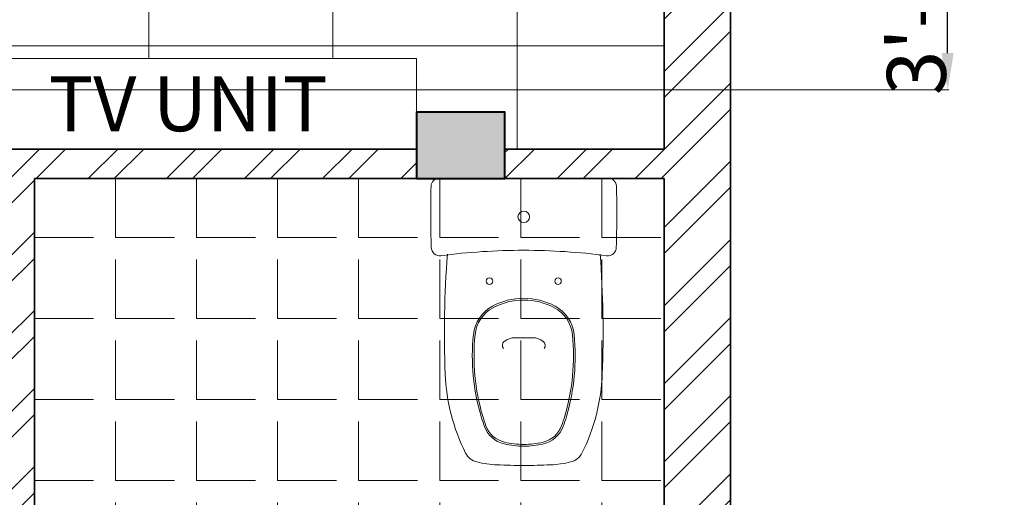
# Model space of a CAD drawing. Units: inches. Extents: x 351 to 1738, y -265 to 286.
# Tile 31 of 38: x 1470 to 1604, y -100 to -35. Entities that reach past the tile are written whole.
import ezdxf

# ---------------------------------------------------------------- set-up
doc = ezdxf.new("R2010")
doc.units = ezdxf.units.IN
doc.header["$MEASUREMENT"] = 0
for name, color, linetype, lineweight in [('A-ANNO-DIMS', 2, 'Continuous', 18), ('A-ANNO-TEXT', 7, 'Continuous', 18), ('A-COLS', 7, 'Continuous', 40), ('A-COLS-PATT', 6, 'Continuous', 13), ('A-FLOR-CASE', 9, 'Continuous', 18), ('A-FLOR-FIXT', 9, 'Continuous', 18), ('A-FLOR-PATT', 9, 'Continuous', 9), ('A-WALL', 7, 'Continuous', 35), ('A-WALL-PATT', 152, 'Continuous', 13)]:
    doc.layers.add(name, color=color, linetype=linetype, lineweight=lineweight)
doc.styles.add('Annotative', font='arial.ttf')
doc.styles.get("Standard").update_dxf_attribs({"font": 'arial.ttf'})
doc.dimstyles.get("Standard").update_dxf_attribs({"dimtxt": 8, "dimasz": 5, "dimexe": 0.18, "dimexo": 0.0625, "dimgap": 0.09, "dimtad": 1, "dimtoh": 1, "dimzin": 0, "dimdsep": 46, "dimlunit": 4, "dimtxsty": 'Standard', "dimcen": 0, "dimclre": 256, "dimadec": 0, "dimazin": 0, "dimtfac": 1, "dimtofl": 0, "dimtmove": 0, "dimatfit": 3, "dimfxl": 1, "dimtolj": 1, "dimtzin": 0, "dimlwe": -1, "dimarcsym": 0})

# ---------------------------------------------------------------- blocks, each defined once
blk = doc.blocks.new('A$C7E916B5A')
for p, q in [((0.019, 0.67), (0.2161, 0.67)), ((0.4133, 0.67), (0.2161, 0.67)), ((0.2161, 0.298), (0.1955, 0.298)), ((0.2161, 0.298), (0.2368, 0.298))]:
    blk.add_line(p, q)
for centre, radius in [((0.2161, 0.58), 0.0135), ((0.1361, 0.43), 0.0075), ((0.2961, 0.43), 0.0075)]:
    blk.add_circle(centre, radius)
for centre, radius, start, end in [((0.019, 0.651), 0.019, 90, 178.4999), ((0.4133, 0.651), 0.019, 1.5001, 90), ((2.5011, 0.586), 2.502, 178.4999, 181.7705), ((-2.0689, 0.586), 2.502, 358.2295, 1.5001), ((0.0203, 0.5093), 0.02, 181.7705, 277.4115), ((0.412, 0.5093), 0.02, 262.5885, 358.2295), ((0.2161, -0.996), 1.498, 90, 97.4115), ((2.5311, 0.3098), 2.5, 175.7895, 182.2108), ((0.2161, -0.996), 1.498, 82.5885, 90), ((-2.0989, 0.3098), 2.5, 357.7892, 4.2105), ((0.1832, 0.2967), 0.085, 118.1012, 174.3336), ((0.1832, 0.2967), 0.081, 118.1012, 174.3336), ((0.2161, 0.235), 0.155, 90, 118.1012), ((0.2161, 0.235), 0.151, 90, 118.1012), ((0.2161, 0.235), 0.155, 61.8988, 90), ((0.2161, 0.235), 0.151, 61.8988, 90), ((0.2491, 0.2967), 0.081, 5.6664, 61.8988), ((0.2491, 0.2967), 0.085, 5.6664, 61.8988), ((0.5961, 0.2558), 0.5, 174.3336, 196.4495), ((0.5961, 0.2558), 0.496, 174.3336, 196.4495), ((-0.1639, 0.2558), 0.496, 343.5505, 5.6664), ((-0.1639, 0.2558), 0.5, 343.5505, 5.6664), ((0.1781, 0.28), 0.012, 128.2132, 217.5723), ((0.1955, 0.258), 0.04, 90, 128.2132), ((0.2368, 0.258), 0.04, 51.7868, 90), ((0.2541, 0.28), 0.012, 322.4277, 51.7868), ((0.4827, 0.2307), 0.45, 182.2108, 206.6241), ((-0.0504, 0.2307), 0.45, 333.3759, 357.7892), ((0.4811, 0.2218), 0.376, 196.4495, 200.1007), ((-0.0488, 0.2218), 0.376, 339.8993, 343.5505), ((0.4811, 0.2218), 0.38, 196.4495, 200.1007), ((0.1851, 0.1135), 0.0609, 200.1007, 256.7352), ((0.2471, 0.1135), 0.0609, 283.2648, 339.8993), ((-0.0488, 0.2218), 0.38, 339.8993, 343.5505), ((0.1851, 0.1135), 0.0649, 200.1007, 256.7352), ((0.2471, 0.1135), 0.0649, 283.2648, 339.8993), ((0.2161, 0.245), 0.2, 256.7352, 270), ((0.2161, 0.245), 0.196, 256.7352, 270), ((0.2161, 0.245), 0.196, 270, 283.2648), ((0.2161, 0.245), 0.2, 270, 283.2648), ((0.1161, 0.047), 0.04, 206.6241, 256.4771), ((0.3161, 0.047), 0.04, 283.5229, 333.3759), ((0.1652, 0.2512), 0.25, 256.477, 267.3481), ((0.2161, 1.35), 1.35, 267.3481, 270), ((0.2161, 1.35), 1.35, 270, 272.6519), ((0.267, 0.2512), 0.25, 272.6519, 283.523)]:
    blk.add_arc(centre, radius, start, end)
blk = doc.blocks.new('CONSOLE-TV')
blk.add_lwpolyline([(0, 0), (61, 0), (61, 12.29), (0, 12.29)], close=True)
blk = doc.blocks.new('COL-9x12')
blk.add_lwpolyline([(0, 12), (0, 0), (9, 0), (9, 12)], close=True)
blk = doc.blocks.new('*D66')
at = {"layer": 'A-ANNO-DIMS', "transparency": 16777216}
for p, q in [((1384.27, -3.5), (1596.33, -3.5)), ((1384.27, -45), (1596.33, -45))]:
    blk.add_line(p, q, dxfattribs=at)
at = {"layer": 'A-ANNO-DIMS', "color": 0, "lineweight": -2, "transparency": 16777216}
blk.add_line((1596.15, -40), (1596.15, -8.5), dxfattribs=at)
at = {"layer": 'A-ANNO-DIMS', "color": 0, "transparency": 16777216}
for points in [[(1595.32, -8.5), (1596.99, -8.5), (1596.15, -3.5)], [(1595.32, -40), (1596.99, -40), (1596.15, -45)]]:
    blk.add_solid(points, dxfattribs=at)
at = {"layer": 'Defpoints', "color": 0, "transparency": 16777216}
for p in [(1384.2, -3.5), (1596.15, -3.5), (1384.2, -45)]:
    blk.add_point(p, dxfattribs=at)
at = {"layer": 'A-ANNO-DIMS', "color": 0, "transparency": 16777216, "insert": (1591.92, -24.25), "char_height": 8, "attachment_point": 5, "rotation": 90}
blk.add_mtext('\\A1;3\'-5 1/2"', dxfattribs=at)

msp = doc.modelspace()

# ---------------------------------------------------------------- hatches: boundary and pattern name
at = {"layer": 'A-COLS-PATT'}
h = msp.add_hatch(color=256, dxfattribs=at)
h.dxf.hatch_style = 1
h.paths.add_polyline_path([(1112.704, 237.963), (1103.704, 237.963), (1103.704, 228.963), (1112.704, 228.963)])
h.paths.add_polyline_path([(1115.704, 237.963), (1112.704, 237.963), (1112.704, 228.963), (1115.704, 228.963)])
h.paths.add_polyline_path([(1043.704, 255.963), (1034.704, 255.963), (1034.704, 243.963), (1043.704, 243.963)])
h.paths.add_polyline_path([(1043.704, 210.963), (1034.704, 210.963), (1034.704, 198.963), (1043.704, 198.963)])
h.paths.add_polyline_path([(1043.704, -45.037), (1034.704, -45.037), (1034.704, -57.037), (1043.704, -57.037)])
h.paths.add_polyline_path([(1112.704, -45.037), (1103.704, -45.037), (1103.704, -57.037), (1112.704, -57.037)])
h.paths.add_polyline_path([(1112.704, -161.037), (1103.704, -161.037), (1103.704, -164.037), (1103.704, -173.037), (1112.704, -173.037)])
h.paths.add_polyline_path([(1043.704, -161.037), (1034.704, -161.037), (1034.704, -173.037), (1043.704, -173.037)])
h.paths.add_polyline_path([(1248.549, -164.037), (1236.549, -164.037), (1236.549, -173.037), (1248.549, -173.037)])
h.paths.add_polyline_path([(1248.549, -50), (1236.549, -50), (1236.549, -59), (1248.549, -59)])
h.paths.add_polyline_path([(1248.704, 73.463), (1244.704, 73.463), (1244.704, 64.463), (1248.704, 64.463)])
h.paths.add_polyline_path([(1244.704, 73.463), (1236.704, 73.463), (1236.704, 64.463), (1244.704, 64.463)])
h.paths.add_polyline_path([(1248.704, 237.963), (1236.704, 237.963), (1236.704, 228.963), (1248.704, 228.963)])
h.paths.add_polyline_path([(1392.204, 237.963), (1380.204, 237.963), (1380.204, 228.963), (1392.204, 228.963)])
h.paths.add_polyline_path([(1536.064, 237.963), (1524.064, 237.963), (1524.064, 228.963), (1536.064, 228.963)])
h.paths.add_polyline_path([(1536.064, 73.463), (1524.064, 73.463), (1524.064, 64.463), (1536.064, 64.463)])
h.paths.add_polyline_path([(1384.204, 73.463), (1380.204, 73.463), (1380.204, 64.463), (1384.204, 64.463)])
h.paths.add_polyline_path([(1392.064, 73.463), (1384.204, 73.463), (1384.204, 64.463), (1392.064, 64.463)])
h.paths.add_polyline_path([(1536.064, -53.037), (1524.064, -53.037), (1524.064, -57.037), (1536.064, -57.037)])
h.paths.add_polyline_path([(1536.064, -48.037), (1524.064, -48.037), (1524.064, -53.037), (1536.064, -53.037)])
h.paths.add_polyline_path([(1392.064, -48.037), (1380.064, -48.037), (1380.064, -56.5), (1380.065, -57.037), (1392.064, -57.037)])
h.paths.add_polyline_path([(1536.064, -164.037), (1524.064, -164.037), (1524.064, -173.037), (1536.064, -173.037)])
at = {"layer": 'A-FLOR-PATT', "transparency": 33554559}
h = msp.add_hatch(dxfattribs=at)
h.set_pattern_fill('ANSI37', color=256, scale=200, angle=135)
h.set_pattern_definition([(180, (1112.704, -164.037), (-2e-15, -25), []), (270, (1112.704, -164.037), (25, -5e-15), [])])
h.paths.add_polyline_path([(1380.064, 73.463), (1380.132, 148.463), (1338.064, 148.463), (1290.704, 148.463), (1290.704, 88.463), (1248.704, 88.463), (1248.704, -2.009), (1244.704, -2.009), (1244.704, 142.457), (1160.704, 142.457), (1160.704, 158.963), (1160.704, 170.137), (1160.704, 206.137), (1160.704, 228.963), (1112.704, 228.963), (1112.704, 209.963), (1112.704, 168.963), (1124.704, 168.963), (1124.704, 162.963), (1112.704, 162.963), (1112.704, 64.463), (1112.704, 60.463), (1112.704, 0.463), (1112.704, -48.026), (1146.804, -47.981), (1146.804, -35.691), (1207.804, -35.691), (1207.804, -47.902), (1236.542, -47.864), (1236.544, -50.009), (1248.5, -50.009), (1248.506, -102.915), (1248.512, -150.915), (1248.514, -164.037), (1248.549, -164.037), (1273.017, -164.037), (1273.017, -128.799), (1355.24, -128.799), (1355.24, -164.037), (1384.204, -164.037), (1384.204, -57.037), (1380.064, -57.037), (1380.064, -48.037), (1392.064, -48.037), (1392.064, -53.037), (1406.549, -53.037), (1406.549, -57.037), (1401.204, -57.037), (1401.204, -147.037), (1468.204, -147.037), (1468.204, -138.5), (1472.204, -138.5), (1472.204, -102.5), (1468.204, -102.5), (1468.204, -57.037), (1442.549, -57.037), (1442.549, -53.037), (1463.049, -53.037), (1463.049, -40.747), (1524.049, -40.747), (1524.049, -48.037), (1536.064, -48.037), (1536.064, -53.037), (1557.704, -53.037), (1557.704, 204.963), (1384.204, 204.963), (1384.204, 73.463), (1392.064, 73.463), (1392.064, 64.463), (1384.204, 64.463), (1384.204, -3.5), (1380.204, -3.537), (1380.204, 64.463), (1380.064, 64.463)])
h.paths.add_polyline_path([(1510.714, 86.458, -0.1039845), (1511.661, 85.595, 0.4704384), (1510.158, 87.614, 0.0961001)], flags=16)
h.paths.add_polyline_path([(1510.443, 100.266, 0.009798), (1504.693, 100.48, 0.0287898), (1504.6, 99.767, -0.1653311), (1505.519, 96.135, -0.1436014)], flags=16)
h.paths.add_polyline_path([(1487.201, 85.595, -0.1039845), (1488.148, 86.458, 0.0961001), (1488.704, 87.614, 0.4704384)], flags=0)
h.paths.add_polyline_path([(1495.052, 100.43), (1494.178, 100.43, -0.0264629), (1494.262, 99.774, -0.1442193)], flags=16)
h.paths.add_polyline_path([(1444.485, 86.458, -0.1039845), (1445.433, 85.595, 0.4704384), (1443.93, 87.614, 0.0961001)], flags=16)
h.paths.add_polyline_path([(1420.972, 85.595, -0.1039845), (1421.92, 86.458, 0.0961001), (1422.475, 87.614, 0.4704384)], flags=16)
h.paths.add_polyline_path([(1428.632, 100.335, 0.0010541), (1427.971, 100.309, -0.0215241), (1428.033, 99.774, -0.1143008)], flags=16)
h.paths.add_polyline_path([(1419.906, 143.708, 0.0249793), (1420.222, 157.526), (1421.573, 159.101), (1421.573, 175.369), (1391.393, 175.369), (1391.393, 200.519), (1542.294, 200.519), (1542.294, 175.369), (1512.028, 175.369, 0.0198653), (1511.521, 153.838, 0.0251335), (1512.758, 118.323, 0.0205529), (1512.942, 115.253), (1419.834, 115.253, -0.0004142), (1419.843, 124.798), (1413.059, 124.798), (1413.059, 84.437, -0.0618528), (1415.831, 80.45, -0.0930773), (1420.972, 85.595, -0.2675367), (1422.371, 84.732, 0.0851103), (1424.052, 84.616, -0.8853927), (1424.033, 84.851, -1.1258145), (1424.073, 84.366, -0.0879871), (1422.371, 84.732, -0.2675367), (1422.326, 83.089, -0.3705421), (1420.972, 85.595, 0.0930773), (1415.831, 80.45, -0.0874142), (1417.914, 73.937), (1418.941, 73.937, 0.0272504), (1418.913, 76.906, -0.1157032), (1421.051, 73.937), (1445.354, 73.937, -0.1157032), (1447.492, 76.906, 0.0272504), (1447.464, 73.937), (1448.491, 73.937, -0.0874142), (1450.574, 80.45, 0.0930773), (1445.433, 85.595, -0.3705421), (1444.079, 83.089, -0.2675367), (1444.034, 84.732, -0.0879871), (1442.332, 84.366, -1.1258145), (1442.372, 84.851, -2.0327363), (1442.364, 84.368, 0.0863779), (1444.034, 84.732, -0.2675367), (1445.433, 85.595, -0.0930773), (1450.574, 80.45, -0.2577317), (1466.483, 90.927, -0.4786702), (1468.832, 91.907, -0.4786702), (1471.18, 90.927, -0.26264), (1483.053, 81.78, -0.0718662), (1487.201, 85.595, -0.2675367), (1488.6, 84.732, 0.0851103), (1490.28, 84.616, -0.8853927), (1490.262, 84.851, -1.1258145), (1490.301, 84.366, -0.0879871), (1488.6, 84.732, -0.2675367), (1488.554, 83.089, -0.3705421), (1487.201, 85.595, 0.0718662), (1483.053, 81.78, -0.1320648), (1484.143, 73.937), (1485.169, 73.937, 0.0272504), (1485.142, 76.906, -0.1157032), (1487.28, 73.937), (1511.582, 73.937, -0.1157032), (1513.72, 76.906, 0.0272504), (1513.693, 73.937), (1514.719, 73.937, -0.0874142), (1516.802, 80.45, 0.0930773), (1511.661, 85.595, -0.3705421), (1510.308, 83.089, -0.2675367), (1510.262, 84.732, -0.0879871), (1508.561, 84.366, -1.1258145), (1508.601, 84.851, -2.0327363), (1508.592, 84.368, 0.0863779), (1510.262, 84.732, -0.2675367), (1511.661, 85.595, -0.0930773), (1516.802, 80.45, -0.0618528), (1519.575, 84.437), (1519.575, 73.937), (1413.059, 73.937), (1413.059, 124.798), (1419.843, 124.798, -0.0008205)], flags=16)
h.paths.add_polyline_path([(1220.149, 54.133, -0.1039845), (1220.869, 53.476, 0.4704384), (1219.727, 55.011, 0.0961001)], flags=16)
h.paths.add_polyline_path([(1219.944, 64.626, 0.009798), (1215.574, 64.789, 0.0287898), (1215.503, 64.247, -0.1653311), (1216.201, 61.487, -0.1436014)], flags=16)
h.paths.add_polyline_path([(1209.779, 64.449, 0.0974459), (1209.339, 64.751), (1208.247, 64.751, 0.1273905), (1207.7, 64.326, 0.1715858), (1206.95, 61.475, -0.1588542), (1207.636, 59.45, 0.0158984), (1207.795, 59.218, 0.0615457), (1208.598, 59.616, 0.1754158), (1208.638, 60.099, -0.2847793), (1209.348, 62.472, 0.3262165)], flags=16)
h.paths.add_polyline_path([(1169.818, 54.133, -0.1039845), (1170.538, 53.476, 0.4704384), (1169.396, 55.011, 0.0961001)], flags=16)
h.paths.add_polyline_path([(1159.017, 62.472, 0.2847642), (1158.307, 60.099, -0.1754332), (1158.267, 59.616, 0.3929302), (1159.448, 64.449, -0.3262298)], flags=16)
h.paths.add_polyline_path([(1156.342, 58.239, -0.1783213), (1154.011, 55.31, -0.1747359), (1154.722, 55.233, -0.2008015), (1156.27, 56.086, 0.1269899), (1157.283, 58.991, -0.0912053)], flags=16)
h.paths.add_polyline_path([(1156.624, 61.413, 0.1572752), (1157.316, 64.247, 0.1696217)], flags=16)
h.paths.add_polyline_path([(1152.67, 54.133, -0.0961001), (1151.95, 53.476, 0.0640762), (1154.465, 54.384, 0.1990158)], flags=16)
h.paths.add_polyline_path([(1202.281, 53.476, -0.1039845), (1203, 54.133, 0.0961001), (1203.423, 55.011, 0.4704384)], flags=0)
h.paths.add_polyline_path([(1151.139, 97.64, 0.0249793), (1151.379, 108.141), (1152.406, 109.338), (1152.406, 121.701), (1129.47, 121.701), (1129.47, 140.814), (1244.149, 140.814), (1244.149, 121.701), (1221.148, 121.701, 0.0198653), (1220.763, 105.338, 0.0251335), (1221.703, 78.349, 0.0205529), (1221.843, 76.016), (1151.078, 76.016, -0.1287433), (1148.786, 65.037, 0.5393525), (1150.327, 64.171, -0.027594), (1163.481, 64.751, 0.0976954), (1163.04, 64.449, 0.3262165), (1163.471, 62.472, -0.2847765), (1164.181, 60.099, -0.1947567), (1165.846, 61.443, -0.1554021), (1165.172, 64.247, -0.1660224), (1165.869, 61.475, -0.1770142), (1167.852, 62.77, -0.4482027), (1169.974, 60.807, -0.3934987), (1167.679, 57.86, -0.8955483), (1168.438, 54.524, -0.3557668), (1166.218, 56.086, -0.066024), (1165.505, 57.539), (1165.251, 56.243, -0.3717324), (1164.02, 59.758, -0.3736141), (1163.04, 64.449, -0.0976954), (1163.481, 64.751, 0.0213538), (1153.294, 64.429, -0.1341826), (1156.695, 61.368, 0.1868727), (1154.636, 62.77, 0.4482027), (1152.514, 60.807, 0.4037263), (1154.905, 57.846, 0.7112192), (1153.334, 55, 0.5315397), (1151.95, 53.476, -0.2675367), (1153.013, 52.821, 0.0851103), (1154.29, 52.732, -0.8853927), (1154.276, 52.911, -1.1258145), (1154.306, 52.543, -0.0879871), (1153.013, 52.821, -0.2675367), (1152.978, 51.572, -0.3705421), (1151.95, 53.476, 0.0930773), (1148.043, 49.566, -0.0874142), (1149.626, 44.617), (1150.406, 44.617, 0.0272504), (1150.385, 46.873, -0.1157032), (1152.01, 44.617), (1170.478, 44.617, -0.1157032), (1172.103, 46.873, 0.0272504), (1172.082, 44.617), (1172.862, 44.617, -0.0874142), (1174.445, 49.566, 0.0930773), (1170.538, 53.476, -0.3705421), (1169.51, 51.572, -0.2675367), (1169.475, 52.821, -0.0879871), (1168.182, 52.543, -1.1258145), (1168.212, 52.911, -2.0327363), (1168.206, 52.544, 0.0863779), (1169.475, 52.821, -0.2675367), (1170.538, 53.476, -0.0930773), (1174.445, 49.566, -0.2577317), (1186.536, 57.528, -0.4786702), (1188.321, 58.273, -0.4786702), (1190.106, 57.528, -0.26264), (1199.128, 50.577, -0.0718662), (1202.281, 53.476, -0.2675367), (1203.344, 52.821, 0.0851103), (1204.621, 52.732, -0.8853927), (1204.607, 52.911, -1.1258145), (1204.637, 52.543, -0.0879871), (1203.344, 52.821, -0.2675367), (1203.309, 51.572, -0.3705421), (1202.281, 53.476, 0.0718662), (1199.128, 50.577, -0.1320648), (1199.957, 44.617), (1200.737, 44.617, 0.0272504), (1200.716, 46.873, -0.1157032), (1202.341, 44.617), (1220.809, 44.617, -0.1157032), (1222.434, 46.873, 0.0272504), (1222.413, 44.617), (1223.193, 44.617, -0.0874142), (1224.776, 49.566, 0.0930773), (1220.869, 53.476, -0.3705421), (1219.841, 51.572, -0.2675367), (1219.806, 52.821, -0.0879871), (1218.513, 52.543, -1.1258145), (1218.543, 52.911, -2.0327363), (1218.537, 52.544, 0.0863779), (1219.806, 52.821, -0.2675367), (1220.869, 53.476, -0.0930773), (1224.776, 49.566, -0.0618528), (1226.883, 52.597), (1226.883, 44.617), (1145.936, 44.617), (1145.936, 83.269), (1151.091, 83.269, -0.0008205)], flags=16)
h.paths.add_polyline_path([(1218.01, 57.86, -0.8955483), (1218.769, 54.524, -0.3557668), (1216.549, 56.086, -0.066024), (1215.836, 57.539), (1215.582, 56.243, -0.3717324), (1214.351, 59.758, -0.3736141), (1213.371, 64.449, 0.3262165), (1213.802, 62.472, -0.2847765), (1214.512, 60.099, -0.1947567), (1216.177, 61.443, -0.1799907), (1218.183, 62.77, -0.4482027), (1220.305, 60.807, -0.3934987)], flags=16)
h.paths.add_polyline_path([(1424.735, 91.363, -0.3934987), (1421.715, 95.241, -0.4482027), (1424.507, 97.824, -0.1799907), (1427.147, 96.077, -0.1947567), (1429.338, 94.309, -0.2847765), (1430.272, 97.432, 0.3262165), (1430.839, 100.034, -0.3736141), (1429.55, 93.861, -0.3717324), (1427.929, 89.235), (1427.596, 90.941, -0.066024), (1426.657, 89.029, -0.3557668), (1423.736, 86.973, -0.8955483)], flags=16)
h.paths.add_polyline_path([(1238.033, 131.257, -1), (1227.329, 131.257, -1)], flags=0)
h.paths.add_polyline_path([(1235.357, 131.257, -1), (1230.005, 131.257, -1)], flags=0)
h.paths.add_polyline_path([(1214.039, 54.243, 0.1543819), (1214.38, 53.992, 0.3589549), (1213.613, 54.016, 0.6039484), (1214.379, 53.657, 0.3713191), (1213.968, 52.872, 0.1879935), (1214.312, 52.809, -0.592455), (1213.953, 52.967, -0.2942791), (1214.083, 53.691, -1.3001871), (1213.881, 54.134, -0.2837621), (1214.469, 53.896, 1.1509396)], flags=16)
h.paths.add_polyline_path([(1212.091, 56.286, -0.4084338), (1211.337, 56.445, -0.0362594), (1211.098, 56.848, -0.2360976), (1211.59, 56.63, 0.0353445), (1211.835, 56.543, -0.4752408), (1212.091, 56.286, -0.4752408), (1212.438, 56.182, 0.0353445), (1212.631, 56.007, -0.2360976), (1213.056, 55.676, -0.0362594), (1212.588, 55.697, -0.4084338)], flags=16)
h.paths.add_polyline_path([(1211.469, 50.297, 0.296043), (1210.47, 50.527, 0.310883), (1211.931, 50.148, 0.0212546)], flags=16)
h.paths.add_polyline_path([(1213.739, 51.818, -0.0362594), (1213.271, 51.838, -0.4084337), (1212.774, 52.427, -0.0947856), (1212.293, 50.703, 1.1504738), (1212.911, 50.232, 0.1662877), (1213.265, 50.68, -0.0252543), (1212.603, 50.13, 1.0879317), (1212.471, 49.407, 0.1662877), (1213.02, 49.251, -0.016128), (1212.567, 49.563, -0.286859), (1212.217, 49.638, 0.0221563), (1212.046, 50.055, -0.6461302), (1212.185, 50.498, 0.0884116), (1212.732, 52.077, -1.1860374), (1213.121, 52.323, 0.0353445), (1213.314, 52.148, -0.2360976)], flags=16)
h.paths.add_polyline_path([(1212.094, 50.342, -0.0485241), (1211.54, 49.605, -1.1038339), (1211.397, 48.738, -0.7855147), (1211.683, 48.254, -0.3920429), (1210.948, 48.525, -0.3928194), (1210.561, 47.995, -0.592455), (1210.201, 48.153, -0.2942791), (1210.331, 48.877, -0.7041716), (1210.316, 49.592, -0.6793441), (1210.729, 50.112, 0.5636764)], flags=16)
h.paths.add_polyline_path([(1211.274, 49.829, -0.1398258), (1210.745, 49.859, -0.2178785), (1210.948, 49.509, -0.4985724)], flags=0)
h.paths.add_polyline_path([(1433.426, 81.49, -0.181571), (1434.245, 81.788, -0.0080665), (1433.726, 82.205, 0.0455784), (1432.755, 81.242, 0.1790113)], flags=16)
h.paths.add_polyline_path([(1434.146, 81.009, -0.1324418), (1433.645, 80.771, 0.2590893), (1433.234, 80.471, -0.1802109), (1433.392, 80.805, -0.1699398), (1432.758, 81.109, 0.0326525), (1433.273, 80.474, -0.4933627), (1434.046, 80.146, -0.3904966)], flags=16)
h.paths.add_polyline_path([(1434.83, 80.047, -0.9475376), (1435.294, 79.576, -0.2991282), (1434.625, 79.404, -0.2704392), (1435.01, 78.591, -0.592455), (1434.537, 78.382, -0.3928194), (1434.027, 79.08, -0.3920429), (1433.06, 78.723, -0.3520423), (1433.003, 79.197, -0.1972159), (1433.75, 79.734, -0.7136405), (1434.447, 79.939, -0.2147903), (1434.819, 80.475, 0.4088333), (1435.075, 80.803, -0.2261519)], flags=16)
h.paths.add_polyline_path([(1432.67, 81.217, -0.4542182), (1431.897, 79.923, -0.4144105), (1431.301, 80.035, 0.0161291), (1431.897, 80.445, 0.2795702), (1432.073, 80.871, -0.2895037), (1431.103, 81.321, -0.4144105), (1430.978, 81.915, 0.0161296), (1431.586, 81.521, 0.341293), (1432.125, 81.583, -0.8131856)], flags=16)
h.paths.add_polyline_path([(1429.893, 86.381, -0.9475376), (1430.358, 85.91, -0.1731062), (1429.984, 85.712, -0.0388172), (1431.625, 84.214, -0.0879005), (1432.097, 88.549, -0.0497684), (1431.254, 88.49, -0.2360976), (1431.814, 88.925, 0.0353445), (1432.067, 89.155, -0.4752408), (1432.524, 89.291, -0.4752408), (1432.86, 89.63, 0.0353445), (1433.182, 89.744, -0.2360976), (1433.83, 90.032, -0.0362594), (1433.516, 89.502, -0.4084338), (1432.524, 89.291, -0.3124239), (1432.106, 88.58, 0.0885594), (1431.625, 84.214, -0.4084337), (1430.971, 83.439, -0.0362594), (1430.355, 83.412, -0.2360976), (1430.914, 83.847, 0.0353445), (1431.168, 84.078, -0.4752408), (1431.625, 84.214, 0.0388172), (1429.984, 85.712, -0.3217316), (1429.333, 86.048, -0.32743), (1429.883, 86.809, 0.4088333), (1430.138, 87.138, -0.2261519)], flags=16)
h.paths.add_polyline_path([(1211.206, 58.616, -0.9997836), (1211.336, 59.323, -0.6149935)], flags=16)
h.paths.add_polyline_path([(1210.288, 49.429, 0.1543819), (1210.629, 49.178, 0.3589549), (1209.861, 49.202, 0.6039484), (1210.627, 48.843, -0.5348247), (1210.806, 49.295, 0.7483464)], flags=16)
h.paths.add_polyline_path([(1209.589, 51.828, -0.0087906), (1209.775, 51.753, 0.1122315), (1209.466, 52.019, 1.4188509), (1209.014, 51.708, -0.4587257), (1208.651, 51.073, -0.592455), (1208.291, 51.232, -0.2942791), (1208.421, 51.955, -1.3001871), (1208.219, 52.398, -0.2260052), (1208.719, 52.257, -0.4755189), (1209.158, 52.369, -1.4554994), (1209.603, 52.664, 0.4213049), (1209.191, 52.262, -0.5912116), (1208.979, 51.796, 0.4973986), (1209.773, 51.333, 0.6493116)], flags=16)
h.paths.add_polyline_path([(1208.029, 52.041, 0.5446671), (1208.832, 52.045, 0.220132)], flags=0)
h.paths.add_polyline_path([(1210.438, 51.425, -0.2041997), (1210.277, 52.018, 0.2708262), (1209.915, 52.897, 0.3241145)], flags=0)
h.paths.add_polyline_path([(1209.668, 52.407, -0.60139), (1208.99, 52.221, -0.3949159), (1208.248, 52.83, -0.8367916), (1208.651, 53.017, -0.3384876), (1209.039, 52.571, 0.1941379), (1209.191, 52.262, 0.4139945), (1209.712, 52.475, 0.5177103), (1210.503, 51.416, 0.401922), (1209.493, 50.93, 0.2063956), (1209.516, 50.165, -0.3194629), (1210.417, 51.418, -0.466635)], flags=16)
h.paths.add_polyline_path([(1206.601, 56.086, -0.3557668), (1204.381, 54.524, -0.9211983), (1205.236, 57.846, 0.2065693), (1207.614, 58.991, -0.1269899)], flags=16)
h.paths.add_polyline_path([(1435.487, 82.816, 0.5277653), (1436.615, 83.361, 0.5085402), (1437.05, 82.433, 0.592455), (1437.524, 82.641, 0.3312448), (1436.963, 83.548, 0.3878632), (1437.808, 83.626, 0.5929544), (1437.618, 84.176, 0.2260158), (1436.961, 83.99, 0.3182053), (1437.588, 84.854, 0.6893744), (1437.05, 84.991, 0.3357648), (1436.539, 84.41, -0.1569934), (1436.404, 84.065, -0.4346112), (1436.961, 83.99, -0.2147903), (1437.333, 84.526, 0.4088333), (1437.588, 84.854, -0.2261519), (1437.343, 84.097, -0.9475376), (1437.808, 83.626, -0.2991282), (1437.139, 83.455, -0.2704392), (1437.524, 82.641, -0.592455), (1437.05, 82.433, -0.3928194), (1436.541, 83.13, -0.4396601), (1435.475, 82.794, -0.174614), (1435.942, 82.244, -0.2063956), (1435.912, 81.237, -0.2708262), (1435.125, 82.208, 0.2079765), (1434.686, 82.904, -0.1964955)], flags=16)
h.paths.add_polyline_path([(1435.386, 84.832, 0.270811), (1434.91, 83.676, -0.2042174), (1434.699, 82.895, 0.3241145)], flags=0)
h.paths.add_polyline_path([(1435.68, 84.18, -0.2176564), (1435.554, 83.304, -0.1767045), (1436.236, 83.778, -0.3730364)], flags=0)
h.paths.add_polyline_path([(1435.566, 100.034, 0.3262165), (1436.133, 97.432, -0.2847765), (1437.067, 94.309, -0.1947567), (1439.258, 96.077, -0.1554021), (1438.371, 99.767, -0.1660224), (1439.289, 96.12, -0.1770142), (1441.897, 97.824, -0.4482027), (1444.69, 95.241, -0.3934987), (1441.67, 91.363, -0.8955483), (1442.669, 86.973, -0.3557668), (1439.748, 89.029, -0.066024), (1438.809, 90.941), (1438.476, 89.235, -0.3717324), (1436.855, 93.861, -0.3736141)], flags=16)
h.paths.add_polyline_path([(1191.252, 49.507, -0.2740221), (1190.658, 48.409, 0.2675367), (1191.311, 47.344, 0.3705421)], flags=0)
h.paths.add_polyline_path([(1190.301, 49.717, 0.1990158), (1188.619, 49.04, 0.0640762), (1191.252, 49.507, -0.0961001)], flags=0)
h.paths.add_polyline_path([(1189.518, 47.857, 1.1258145), (1189.676, 47.523, 2.0446052)], flags=0)
h.paths.add_polyline_path([(1464.974, 80.372, 0.2740221), (1465.756, 78.927, -0.0830131)], flags=0)
h.paths.add_polyline_path([(1464.974, 80.372, 0.3705421), (1464.897, 77.525, 0.5763244)], flags=0)
h.paths.add_polyline_path([(1464.974, 80.372, -0.4704384), (1467.284, 81.372, -0.0961001), (1466.226, 80.648, -0.1990158), (1468.439, 79.757, -0.0640762)], flags=0)
h.paths.add_polyline_path([(1189.511, 56.43, -0.2594668), (1188.321, 56.391, -0.2594668), (1187.13, 56.43, 0.0851103), (1188.193, 55.716, -0.8853927), (1188.27, 55.878, -1.1960133), (1188.355, 55.442, 0.1014587)], flags=0)
h.paths.add_polyline_path([(1188.321, 57.596, 0.0780722), (1187.678, 57.24, 0.0155503), (1188.321, 57.136, 0.0155503), (1188.964, 57.24, 0.0780722)], flags=0)
h.paths.add_polyline_path([(1190.164, 55.365, -0.5763244), (1190.106, 57.528, -0.1982945), (1188.321, 58.319, -0.1982945), (1186.536, 57.528, -0.5763244), (1186.477, 55.365, -0.3705421), (1186.536, 57.528, 0.1982945), (1188.321, 58.319, 0.1982945), (1190.106, 57.528, -0.3705421)], flags=0)
h.paths.add_polyline_path([(1188.372, 55.878, 1.1258145), (1188.529, 55.544, 2.0446052)], flags=0)
h.paths.add_polyline_path([(1186.341, 49.717, -0.0961001), (1185.389, 49.507, 0.0640762), (1188.022, 49.04, 0.1990158)], flags=0)
h.paths.add_polyline_path([(1185.389, 49.507, -0.2675367), (1185.984, 48.409, 0.0851103), (1187.046, 47.695, -0.8853927), (1187.123, 47.857, -1.1258145), (1186.966, 47.523, -0.0879871), (1185.984, 48.409, -0.2675367), (1185.331, 47.344, -0.3705421)], flags=0)
h.paths.add_polyline_path([(1399.441, 187.944, -1), (1413.525, 187.944, -1)], flags=0)
h.paths.add_polyline_path([(1402.962, 187.944, -1), (1410.004, 187.944, -1)], flags=0)
h.paths.add_polyline_path([(1357.663, -72.245), (1377.272, -72.245), (1377.272, -91.854), (1357.663, -91.854)], flags=16)
h.paths.add_polyline_path([(1467.256, 78.201, -1.1258145), (1467.049, 77.761, -2.0446052)], flags=0)
h.paths.add_polyline_path([(1468.822, 88.714, 0.9411249), (1469.106, 88.316, 1.1371523), (1468.765, 88.755, 0.890986), (1468.99, 88.245, 0.0948283), (1470.398, 89.481, -0.2675367), (1471.18, 90.927, -0.0281232), (1469.678, 90.547, -0.0287737), (1469.948, 90.311, -0.0203267), (1468.832, 90.41, -0.0203267), (1467.716, 90.311, -0.0287737), (1467.986, 90.547, -0.0281232), (1466.483, 90.927, -0.2675367), (1467.265, 89.481, 0.0851103), (1468.663, 88.542, -1.2023159)], flags=0)
h.paths.add_polyline_path([(1178.25, 124.523, -0.1199286), (1165.65, 124.145, -0.1073492), (1159.133, 124.446, -0.1028906), (1159.132, 130.465, -0.0748968), (1158.993, 137.956, 0.002027), (1167.844, 137.479, -0.07553), (1180.337, 137.666, -0.0758613), (1186.502, 137.688, -0.1409896), (1186.272, 130.046, -0.0954805), (1186.729, 124.748, -0.10603)], flags=0)
h.paths.add_polyline_path([(1469.225, 79.757, -0.1990158), (1471.437, 80.648, -0.0961001), (1470.379, 81.372, -0.4704384), (1472.689, 80.372, -0.3705421), (1472.766, 77.525, -0.2675367), (1471.907, 78.927, -0.0879863), (1470.615, 77.761, -1.1258491), (1470.408, 78.201, -2.0327363), (1470.642, 77.778, 0.0863779), (1471.907, 78.927, -0.2675367), (1472.689, 80.372, -0.0640762)], flags=0)
h.paths.add_polyline_path([(1430.423, 186.902, -0.0748968), (1430.24, 196.758, 0.002027), (1441.887, 196.131, -0.07553), (1458.326, 196.377, -0.0758613), (1466.438, 196.406, -0.1409896), (1466.136, 186.35, -0.0954805), (1466.737, 179.378, -0.10603), (1455.58, 179.082, -0.1199286), (1439, 178.585, -0.1073492), (1430.425, 178.981, -0.1028906)], flags=0)
h.paths.add_polyline_path([(1162.258, 49.939, 0.3357645), (1161.87, 49.497, -0.1569936), (1161.767, 49.235, -0.4346112), (1162.19, 49.178, -0.2147903), (1162.473, 49.585, 1.5291948)], flags=16)
h.paths.add_polyline_path([(1161.683, 49.021, 0.5815181), (1161.268, 49.583, 0.5927609)], flags=16)
h.paths.add_polyline_path([(1162.602, 48.058, 0.3713191), (1162.192, 48.843, 0.4345332), (1162.88, 48.962, 0.1850806), (1162.197, 48.926, 1.1218369)], flags=16)
h.paths.add_polyline_path([(1161.443, 48.941, -1.3071038), (1161.495, 48.571, -0.2177521), (1161.136, 48.254, 0.6973029), (1161.871, 49.048, 0.1215141)], flags=16)
h.paths.add_polyline_path([(1162.531, 49.429, -0.2070837), (1162.05, 49.146, -0.9920299)], flags=16)
h.paths.add_polyline_path([(1161.304, 49.578, -0.7196675), (1161.513, 50.079, -0.1304275), (1160.836, 50.168, 0.0395926)], flags=0)
h.paths.add_polyline_path([(1162.036, 50.584, -0.0080665), (1161.642, 50.9, 0.0293675), (1161.35, 50.297, -0.2057884)], flags=16)
h.paths.add_polyline_path([(1162.882, 51.392, -0.1247327), (1162.763, 51.828, -0.1011907), (1162.399, 51.438, -0.153425)], flags=0)
h.paths.add_polyline_path([(1164.235, 51.85, -0.3091075), (1164.513, 51.136, -0.6271245), (1163.781, 51.603, -0.6859091), (1162.777, 51.219, -0.2332851), (1163.303, 50.165, -0.2708262), (1162.705, 50.903, 0.2041997), (1162.381, 51.425, 0.204182), (1162.542, 52.018, -0.2708414), (1162.903, 52.897, -0.1272607), (1163.219, 52.529, -1.1686811), (1163.781, 52.587, -0.3291117), (1164.168, 53.017, -0.8367917), (1164.571, 52.83, -0.1933406), (1164.391, 52.338, -0.9475376), (1164.744, 51.981, -0.2991282)], flags=16)
h.paths.add_polyline_path([(1163.598, 51.937, -1.2629561), (1163.236, 51.831, 0.0125754), (1162.971, 51.721, 0.2306566), (1163.151, 52.407, -0.1648982), (1163.178, 52.661, -0.4493201), (1163.628, 52.262, -0.721477), (1164.154, 52.088, -0.8499982)], flags=0)
h.paths.add_polyline_path([(1161.613, 58.616, -0.9804131), (1161.525, 59.049, -2.9089348)], flags=16)
h.paths.add_polyline_path([(1160.252, 49.166, -0.4144105), (1159.799, 49.251, 0.0161291), (1160.252, 49.563, 0.2795702), (1160.386, 49.887, -0.2895037), (1159.649, 50.229, -0.4144105), (1159.554, 50.68, 0.0161296), (1160.015, 50.381, 0.6178854), (1160.526, 50.703, -0.0947856), (1160.045, 52.427, -0.1404436), (1159.682, 52.042, -0.0578559), (1159.3, 51.872, 0.5448433), (1160.046, 52.419, -0.0881216), (1160.404, 55.721, -0.0497684), (1159.763, 55.676, -0.2360976), (1160.188, 56.007, 0.0353445), (1160.381, 56.182, -0.4752408), (1160.728, 56.286, -0.4752408), (1160.984, 56.543, 0.0353445), (1161.229, 56.63, -0.2360976), (1161.721, 56.848, -0.0362594), (1161.482, 56.445, -0.4084338), (1160.728, 56.286, -0.3124239), (1160.411, 55.745, 0.0885594), (1160.045, 52.427, 0.1070813), (1160.634, 50.498, -0.4947977), (1160.839, 50.149, -0.4542182)], flags=16)
h.paths.add_polyline_path([(1160.666, 49.808, -2.0765276), (1160.828, 50.172, 0.0195861)], flags=0)
h.paths.add_polyline_path([(1158.439, 53.992, 0.1543819), (1158.78, 54.243, 0.7483463), (1158.262, 54.109, -0.3382251), (1158.492, 53.839, -0.1708158), (1159.124, 53.779, 0.4957286), (1158.938, 54.134, 0.2260157)], flags=16)
h.paths.add_polyline_path([(1160.045, 52.427, 0.0388172), (1158.798, 53.565, -0.1198178), (1158.574, 53.586, -0.3091075), (1158.851, 52.872, -0.1879935), (1158.506, 52.809, 0.592455), (1158.866, 52.967, 0.3312448), (1158.44, 53.657, 0.2012451), (1158.798, 53.565, -0.034023), (1159.901, 52.578, -0.0442527), (1159.698, 52.323, -0.4752408)], flags=16)
h.paths.add_polyline_path([(1336.926, -95.392), (1336.926, -117.945), (1291.82, -117.945), (1291.82, -95.392)], flags=16)
h.paths.add_polyline_path([(1357.535, -97.244), (1357.726, -96.697, 0.0348443)], flags=16)
h.paths.add_polyline_path([(1376.693, -96.478), (1377.301, -96.5, 0.0314968), (1375.907, -96.424), (1357.726, -96.424)], flags=16)
h.paths.add_polyline_path([(1379.403, -119.667, 0.0267056), (1380.043, -119.439, -0.0152991)], flags=16)
h.paths.add_polyline_path([(1357.726, -120.202), (1357.821, -120.202), (1357.821, -120.201)], flags=16)
h.paths.add_polyline_path([(1354.171, -104.592), (1354.469, -98.672, 0.0111377)], flags=16)
h.paths.add_polyline_path([(1355.058, -119.136), (1354.578, -118.539, 0.1431635)], flags=16)
h.paths.add_polyline_path([(1378.851, -96.821), (1378.85, -96.82), (1378.85, -96.82, -0.0496798), (1380.055, -97.191), (1378.85, -96.82, 0.1500541), (1375.135, -97.188), (1375.136, -119.44, -0.0099698), (1374.747, -116.649), (1357.726, -116.649, 0.1693849), (1357.535, -119.382), (1357.535, -119.382), (1357.535, -119.382, 0.0348176), (1357.726, -119.928), (1357.726, -119.928), (1357.726, -119.929, -0.0348772), (1357.535, -119.382), (1355.507, -119.382), (1355.317, -119.278), (1357.535, -119.382, -0.1693939), (1357.726, -116.649, -0.0391513), (1374.686, -116.113, -0.0020149), (1374.625, -115.546, 0.1153223), (1369.915, -115.474, 0.0609215), (1369.922, -101.154, 0.1151459), (1374.625, -101.079, -0.0020164), (1374.686, -100.513, -0.0391511), (1357.726, -99.977), (1374.747, -99.977, -0.0099633), (1375.135, -97.188), (1375.135, -97.188, -0.1501081)], flags=16)
h.paths.add_polyline_path([(1490.963, 91.363, -0.3934987), (1487.944, 95.241, -0.4482027), (1490.736, 97.824, -0.1799907), (1493.376, 96.077, -0.1947567), (1495.567, 94.309, -0.2847765), (1496.501, 97.432, 0.3262165), (1497.068, 100.034, -0.3736141), (1495.778, 93.861, -0.3717324), (1494.158, 89.235), (1493.824, 90.941, -0.066024), (1492.886, 89.029, -0.3557668), (1489.964, 86.973, -0.8955483)], flags=16)
h.paths.add_polyline_path([(1354.86, -97.658), (1355.316, -97.348, 0.1019112)], flags=16)
h.paths.add_polyline_path([(1497.063, 83.327, 0.1767244), (1496.37, 83.785, -0.4051388), (1496.016, 83.384, 0.4973986), (1497.06, 82.774, 0.6493116), (1496.818, 83.426, -0.0087906)], flags=16)
h.paths.add_polyline_path([(1496.339, 83.783, 0.5927609), (1496.886, 84.522, 0.5815181)], flags=16)
h.paths.add_polyline_path([(1495.11, 82.641, 0.592455), (1495.583, 82.433, 0.6769152), (1495.805, 83.59, 0.3756693)], flags=16)
h.paths.add_polyline_path([(1495.015, 84.176, -0.145057), (1495.301, 84.526, -0.4088333), (1495.045, 84.854, 0.2206292), (1495.381, 84.152, -0.199594), (1495.851, 83.764, -0.5240172), (1494.826, 83.626, -0.5929976)], flags=16)
h.paths.add_polyline_path([(1501.655, 81.915, -0.0161291), (1501.048, 81.521, -0.3927187), (1500.462, 81.37, -0.2106699), (1500.607, 81.142, 0.3066994)], flags=16)
h.paths.add_polyline_path([(1500.11, 89.291, -0.4084338), (1499.118, 89.502, -0.0362594), (1498.803, 90.032, -0.2360976), (1499.451, 89.744, 0.0353445), (1499.774, 89.63, -0.4752408), (1500.11, 89.291, -0.4752408), (1500.567, 89.155, 0.0353445), (1500.82, 88.925, -0.2360976), (1501.379, 88.49, -0.0362594), (1500.763, 88.516, -0.4084338)], flags=16)
h.paths.add_polyline_path([(1498.908, 82.205, -0.0513217), (1500.013, 81.134, -0.5879306), (1500.234, 81.676, 0.1070813), (1501.009, 84.214, -0.03529)], flags=16)
h.paths.add_polyline_path([(1496.93, 83.875, -0.2063956), (1497.247, 84.832, -0.2708262), (1497.724, 83.676, 0.2079765), (1497.944, 82.884, -0.3814554)], flags=16)
h.paths.add_polyline_path([(1496.721, 81.237, 0.2708125), (1497.509, 82.208, -0.2042157), (1497.935, 82.895, 0.3241145)], flags=16)
h.paths.add_polyline_path([(1497.529, 80.125, -0.145057), (1497.814, 80.475, -0.703182), (1498.282, 81.178, -0.1229248), (1497.977, 81.714, -0.2708368), (1499.207, 81.49, 0.2079641), (1499.993, 81.248, -0.2651454), (1499.278, 80.472, 0.3819006), (1498.808, 79.947, -0.3059049), (1498.848, 79.519, 0.4994816), (1498.574, 79.217, -0.4587257), (1498.097, 78.382, -0.592455), (1497.624, 78.591, -0.2704392), (1498.009, 79.404, -0.299116), (1497.34, 79.576, -0.5930157)], flags=16)
h.paths.add_polyline_path([(1500.736, 79.923, 0.4144105), (1501.333, 80.035, -0.3216484), (1500.192, 80.765, 0.0198856), (1499.976, 81.251, 0.4653307)], flags=16)
h.paths.add_polyline_path([(1501.009, 84.214, -0.0388172), (1502.649, 85.712, -0.1730946), (1502.276, 85.91, -0.5930157), (1502.465, 86.46, -0.145057), (1502.751, 86.809, -0.4088333), (1502.495, 87.138, 0.2206292), (1502.831, 86.436, -0.199594), (1503.301, 86.048, -0.3217316), (1502.649, 85.712, 0.0388172), (1501.009, 84.214, 0.1224486), (1501.412, 83.755, 0.4754908), (1501.335, 84.226, 0.055822), (1501.719, 83.847, -0.2360976), (1502.278, 83.412, -0.0362594), (1501.663, 83.439, -0.4084338)], flags=16)
h.paths.add_polyline_path([(1501.794, 100.034, 0.3262165), (1502.362, 97.432, -0.2847765), (1503.295, 94.309, -0.1947567), (1505.486, 96.077, -0.1799907), (1508.126, 97.824, -0.4482027), (1510.918, 95.241, -0.3934987), (1507.899, 91.363, -0.8955483), (1508.898, 86.973, -0.3557668), (1505.976, 89.029, -0.066024), (1505.038, 90.941), (1504.704, 89.235, -0.3717324), (1503.084, 93.861, -0.3736141)], flags=16)
h.paths.add_polyline_path([(1146.29, 131.257, -1), (1135.587, 131.257, -1)], flags=0)
h.paths.add_polyline_path([(1143.614, 131.257, -1), (1138.262, 131.257, -1)], flags=0)
h.paths.add_polyline_path([(1524.064, 73.463), (1536.064, 73.463), (1536.064, 64.463), (1524.064, 64.463)], flags=16)
h.paths.add_polyline_path([(1520.162, 187.944, -1), (1534.246, 187.944, -1)], flags=0)
h.paths.add_polyline_path([(1530.725, 187.944), (1527.204, 187.944), (1527.204, 184.423, 0.4142136)], flags=0)
h.paths.add_polyline_path([(1278.415, -91.154), (1331.067, -91.154), (1331.067, -80.583), (1278.415, -80.583)], flags=24)
h.paths.add_polyline_path([(1266.655, -79.354), (1354.738, -79.354), (1354.738, -67.817), (1266.655, -67.817)], flags=24)
h.paths.add_polyline_path([(1115.482, 206.184), (1155.098, 206.184), (1155.098, 217.714), (1115.482, 217.714)], flags=24)
h.paths.add_polyline_path([(1161.771, 8.501), (1222.466, 8.501), (1222.466, 19.079), (1161.771, 19.079)], flags=24)
h.paths.add_polyline_path([(1164.656, 18.795), (1210.615, 18.795), (1210.615, 30.324), (1164.656, 30.324)], flags=24)
h.paths.add_polyline_path([(1368.147, -32.882), (1379.362, -32.882), (1379.362, -21.733), (1368.147, -21.733)], flags=24)
h.paths.add_polyline_path([(1244.842, -31.012), (1256.057, -31.012), (1256.057, -19.863), (1244.842, -19.863)], flags=24)
h.paths.add_polyline_path([(1114.589, 195.739), (1156.517, 195.739), (1156.517, 206.31), (1114.589, 206.31)], flags=24)
h.paths.add_polyline_path([(1436.398, 37.632), (1505.131, 37.632), (1505.131, 48.203), (1436.398, 48.203)], flags=24)
h.paths.add_polyline_path([(1435.991, 47.919), (1507.906, 47.919), (1507.906, 59.456), (1435.991, 59.456)], flags=24)
h.paths.add_polyline_path([(1415.107, -124.896), (1457.038, -124.896), (1457.038, -114.318), (1415.107, -114.318)], flags=24)
h.paths.add_polyline_path([(1417.992, -114.602), (1457.609, -114.602), (1457.609, -103.073), (1417.992, -103.073)], flags=24)
at = {"layer": 'A-FLOR-PATT', "transparency": 33554610}
h = msp.add_hatch(dxfattribs=at)
h.set_pattern_fill('ANGLE', color=256, scale=40)
h.set_pattern_definition([(0, (1472.204, -164.037), (0, 11), [8, -3]), (90, (1472.204, -164.037), (-11, 7e-16), [8, -3])])
h.paths.add_polyline_path([(1557.704, -57.037), (1472.204, -57.037), (1472.204, -102.5), (1472.204, -138.5), (1472.204, -164.037), (1557.704, -164.037)])
at = {"layer": 'A-WALL-PATT'}
h = msp.add_hatch(dxfattribs=at)
h.set_pattern_fill('ANSI32', color=256, scale=20)
h.set_pattern_definition([(45, (1034.704, -173.037), (-5.3033, 5.3033), []), (45, (1038.24, -173.037), (-5.3033, 5.3033), [])])
h.paths.add_polyline_path([(1043.704, -57.037), (1034.704, -57.037), (1034.704, -81.037), (1043.704, -81.037)])
h.paths.add_polyline_path([(1043.704, 198.963), (1034.704, 198.963), (1034.704, -45.037), (1043.704, -45.037)])
h.paths.add_polyline_path([(1043.704, 243.963), (1034.704, 243.963), (1034.704, 237.963), (1034.704, 210.963), (1043.704, 210.963)])
h.paths.add_polyline_path([(1112.704, 255.963), (1043.704, 255.963), (1043.704, 246.963), (1103.704, 246.963), (1103.704, 237.963), (1112.704, 237.963), (1112.704, 251.963)])
h.paths.add_polyline_path([(1056.704, 207.963), (1043.704, 207.963), (1043.704, 198.963), (1056.704, 198.963)])
h.paths.add_polyline_path([(1103.704, 207.963), (1092.704, 207.963), (1092.704, 198.963), (1103.704, 198.963)])
h.paths.add_polyline_path([(1112.704, 228.963), (1103.704, 228.963), (1103.704, 74.963), (1112.704, 74.963), (1112.704, 97.5)])
h.paths.add_polyline_path([(1284.129, -164.037), (1248.549, -164.037), (1248.549, -173.037), (1284.129, -173.037)])
h.paths.add_polyline_path([(1524.064, -164.037), (1472.204, -164.037), (1472.204, -138.5), (1468.204, -138.5), (1468.204, -164.037), (1344.129, -164.037), (1344.129, -173.037), (1524.064, -173.037)])
h.paths.add_polyline_path([(1384.204, -57.037), (1380.065, -57.037), (1380.204, -164.037), (1384.204, -164.037)])
h.paths.add_polyline_path([(1566.704, -138), (1557.704, -138), (1557.704, -164.037), (1536.064, -164.037), (1536.064, -173.037), (1566.704, -173.037)])
h.paths.add_polyline_path([(1566.704, -30.189), (1557.704, -30.189), (1557.704, -53.037), (1536.064, -53.037), (1536.064, -57.037), (1557.704, -57.037), (1557.704, -102), (1566.704, -102)])
h.paths.add_polyline_path([(1524.064, -53.037), (1442.549, -53.037), (1442.549, -57.037), (1468.204, -57.037), (1468.204, -102.5), (1472.204, -102.5), (1472.204, -57.037), (1524.064, -57.037)])
h.paths.add_polyline_path([(1566.704, 120.993), (1557.704, 120.993), (1557.704, 29.811), (1566.704, 29.811)])
h.paths.add_polyline_path([(1384.204, 64.463), (1380.204, 64.463), (1380.204, -3.5), (1384.204, -3.5)])
h.paths.add_polyline_path([(1266.549, 237.963), (1248.704, 237.963), (1248.704, 228.963), (1266.549, 228.963)])
h.paths.add_polyline_path([(1329.549, 237.963), (1302.549, 237.963), (1302.549, 228.963), (1329.549, 228.963)])
h.paths.add_polyline_path([(1380.204, 237.963), (1365.549, 237.963), (1365.549, 228.963), (1380.204, 228.963)])
h.paths.add_polyline_path([(1524.064, 237.963), (1392.204, 237.963), (1392.204, 228.963), (1524.064, 228.963)])
h.paths.add_polyline_path([(1384.204, 228.963), (1380.204, 228.963), (1380.204, 73.463), (1384.204, 73.463)])
h.paths.add_polyline_path([(1566.704, 237.963), (1536.064, 237.963), (1536.064, 228.963), (1557.704, 228.963), (1557.704, 180.993), (1566.704, 180.993)])

# ---------------------------------------------------------------- linework, layer by layer
at = {"layer": 'A-WALL'}
for p, q in [((1566.704, -173.037), (1566.704, 237.963)), ((1557.704, -53.037), (1557.704, 228.963)), ((1442.549, -53.037), (1524.064, -53.037)), ((1536.064, -53.037), (1557.704, -53.037)), ((1472.204, -57.037), (1557.704, -57.037)), ((1472.204, -57.037), (1472.204, -102.5)), ((1557.704, -164.037), (1557.704, -57.037))]:
    msp.add_line(p, q, dxfattribs=at)

# ---------------------------------------------------------------- block references
at = {"layer": 'A-COLS', "rotation": 90.00000000000007}
msp.add_blockref('COL-9x12', (1536.064, -57.038), dxfattribs=at)
at = {"layer": 'A-FLOR-CASE'}
msp.add_blockref('CONSOLE-TV', (1463.049, -53.037), dxfattribs=at)
at = {"layer": 'A-FLOR-FIXT', "xscale": 58.19959361425425, "yscale": 58.19959361425425, "zscale": 58.19959361425425}
msp.add_blockref('A$C7E916B5A', (1526.049, -96), dxfattribs=at)

# ---------------------------------------------------------------- texts
at = {"layer": 'A-ANNO-TEXT', "style": 'Annotative'}
msp.add_text('TV UNIT', height=7.4326, dxfattribs=at).set_placement((1474.125, -50.615))

# ---------------------------------------------------------------- dimensions: what is measured, and where the dimension line sits
at = {"layer": 'A-ANNO-DIMS'}
dim = msp.add_linear_dim(base=(1596.154, -3.5), p1=(1384.204, -45), p2=(1384.204, -3.5), angle=90, dimstyle='Standard', override={"dimdec": 1, "dimlfac": 1, "dimrnd": 0, "dimzin": 1, "dimdsep": 46, "dimlunit": 4, "dimfrac": 2}, dxfattribs=at)
dim.commit()
dim.dimension.update_dxf_attribs({"geometry": '*D66', "text_midpoint": (1591.925, -24.25)})

doc.saveas('drawing.dxf')
